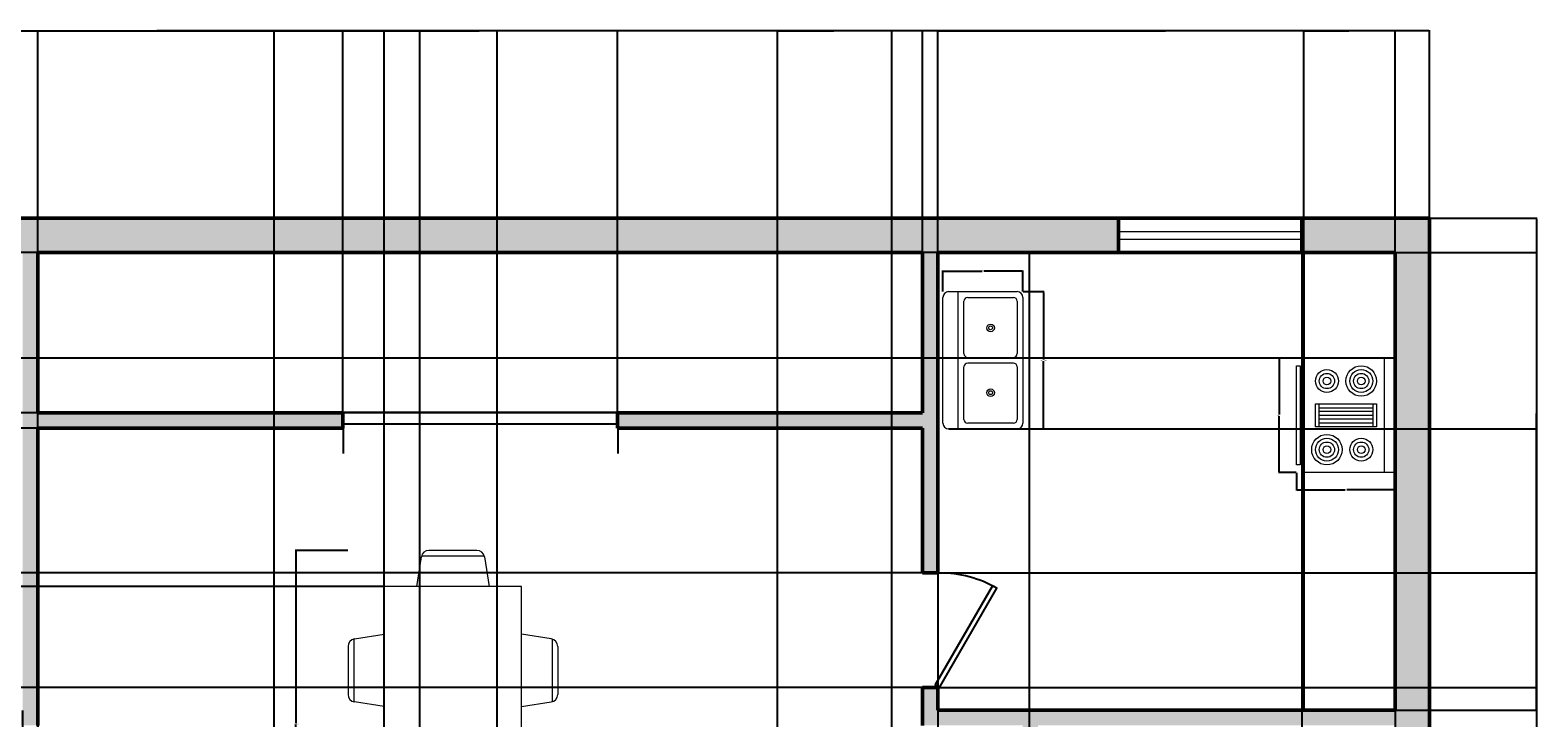
# Model space of a CAD drawing. Units: inches. Extents: x 1869 to 2483, y 2084 to 2479.
# Tile 7 of 7: x 2088 to 2483, y 2299 to 2479. Entities that reach past the tile are written whole.
import ezdxf

# ---------------------------------------------------------------- set-up
doc = ezdxf.new("R2010")
doc.units = ezdxf.units.IN
for name, color, linetype, lineweight in [('A-ANNO-DIMS', 2, 'Continuous', 18), ('A-DOOR', 3, 'Continuous', 25), ('A-EQPM', 8, 'Continuous', 18), ('A-FLOR-CASE', 9, 'Continuous', 25), ('A-FLOR-FIXT', 9, 'Continuous', 18), ('A-FURN', 8, 'Continuous', 18), ('A-GLAZ', 4, 'Continuous', 18), ('A-WALL', 7, 'Continuous', 50)]:
    doc.layers.add(name, color=color, linetype=linetype, lineweight=lineweight)
doc.layers.add('A-WALL-PATT', color=18, linetype='Continuous', lineweight=13, true_color=0x000000)
doc.styles.get("Standard").update_dxf_attribs({"font": 'arial.ttf'})
doc.dimstyles.get("Standard").update_dxf_attribs({"dimtxt": 0.18, "dimasz": 0.18, "dimexe": 0.18, "dimexo": 0.0625, "dimgap": 0.09, "dimtad": 0, "dimtih": 1, "dimtoh": 1, "dimdec": 4, "dimzin": 0, "dimdsep": 46, "dimtxsty": 'Standard', "dimcen": 0.09, "dimadec": 0, "dimazin": 0, "dimtfac": 1, "dimtdec": 4, "dimtofl": 0, "dimtmove": 0, "dimatfit": 3, "dimfxl": 1, "dimtolj": 1, "dimtzin": 0, "dimarcsym": 0})

# ---------------------------------------------------------------- blocks, each defined once
blk = doc.blocks.new('Dining Set - 36 x 72 in.')
for p, q in [((-22.26, 25.81), (-23.48, 18)), ((-22.23, 26), (-5.76, 26)), ((-20.29, 27.5), (-7.71, 27.5)), ((-4.52, 18), (-5.74, 25.81)), ((5.74, 25.81), (4.52, 18)), ((5.77, 26), (22.24, 26)), ((7.71, 27.5), (20.29, 27.5)), ((23.48, 18), (22.26, 25.81)), ((36, 18), (-36, 18)), ((-36, 18), (-36, -18)), ((36, -18), (36, 18)), ((-44, 8.23), (-44, -8.24)), ((-43.81, 8.26), (-36, 9.48)), ((43.81, 8.26), (36, 9.48)), ((44, 8.23), (44, -8.24)), ((-45.5, 6.29), (-45.5, -6.29)), ((45.5, 6.29), (45.5, -6.29)), ((-36, -9.48), (-43.81, -8.26)), ((36, -9.48), (43.81, -8.26)), ((-36, -18), (36, -18)), ((-22.26, -25.81), (-23.48, -18)), ((-4.52, -18), (-5.74, -25.81)), ((5.74, -25.81), (4.52, -18)), ((23.48, -18), (22.26, -25.81)), ((-22.23, -26), (-5.76, -26)), ((-20.29, -27.5), (-7.71, -27.5)), ((5.77, -26), (22.24, -26)), ((7.71, -27.5), (20.29, -27.5))]:
    blk.add_line(p, q)
for centre, start, end in [((-20.29, 25.5), 90, 171.1198), ((-7.71, 25.5), 8.881, 90), ((7.71, 25.5), 90, 171.1198), ((20.29, 25.5), 8.881, 90), ((-43.5, 6.29), 98.8806, 180), ((43.5, 6.29), 0, 81.1194), ((-43.5, -6.29), 180, 261.1194), ((43.5, -6.29), 278.8806, 0), ((-20.29, -25.5), 188.8802, 270), ((-7.71, -25.5), 270, 351.1191), ((7.71, -25.5), 188.8802, 270), ((20.29, -25.5), 270, 351.1191)]:
    blk.add_arc(centre, 2, start, end)
blk = doc.blocks.new('Range-Oven - 30 in top')
for p, q in [((0, -3), (30, -3)), ((12, -6), (18, -6)), ((13, -20), (13, -6)), ((14, -6), (14, -20)), ((15, -20), (15, -6)), ((16, -6), (16, -20)), ((17, -20), (17, -6)), ((18, -20), (12, -20)), ((6, -24), (6, -25)), ((8, -25), (8, -24)), ((22, -25), (22, -24)), ((24, -24), (24, -25))]:
    blk.add_line(p, q)
for points in [[(0, -24), (0, 0), (30, 0), (30, -24)], [(12, -21), (12, -5), (18, -5), (18, -21)], [(2, -26), (2, -25), (28, -25), (28, -26)]]:
    blk.add_lwpolyline(points, close=True)
for centre, radius in [((6, -9), 4), ((6, -9), 3), ((6, -9), 2), ((24, -9), 3), ((24, -9), 2), ((6, -9), 1), ((24, -9), 1), ((6, -18), 3), ((24, -18), 4), ((24, -18), 3), ((6, -18), 2), ((6, -18), 1), ((24, -18), 2), ((24, -18), 1)]:
    blk.add_circle(centre, radius)
blk = doc.blocks.new('Sink-double - 36 in top')
for p, q in [((-18, -4), (18, -4)), ((-0.75, -18.5), (-0.75, -6.5)), ((0.75, -6.5), (0.75, -18.5))]:
    blk.add_line(p, q)
for points in [[(-16.5, 0), (16.5, 0)], [(-18, -19.5), (-18, -1.5)], [(18, -1.5), (18, -19.5)], [(-16.5, -18.5), (-16.5, -6.5)], [(-15.5, -5.5), (-1.75, -5.5)], [(1.75, -5.5), (15.5, -5.5)], [(16.5, -6.5), (16.5, -18.5)], [(-1.75, -19.5), (-15.5, -19.5)], [(15.5, -19.5), (1.75, -19.5)], [(16.5, -21), (-16.5, -21)]]:
    blk.add_lwpolyline(points)
for centre, radius in [((-8.5, -12.5), 1), ((8.5, -12.5), 1), ((-8.5, -12.5), 0.5), ((8.5, -12.5), 0.5)]:
    blk.add_circle(centre, radius)
for centre, radius, start, end in [((-16.5, -1.5), 1.5, 90, 180), ((16.5, -1.5), 1.5, 0, 90), ((-15.5, -6.5), 1, 90, 180), ((-1.75, -6.5), 1, 0, 90), ((1.75, -6.5), 1, 90, 180), ((15.5, -6.5), 1, 0, 90), ((-16.5, -19.5), 1.5, 180, 270), ((-15.5, -18.5), 1, 180, 270), ((-1.75, -18.5), 1, 270, 0), ((1.75, -18.5), 1, 180, 270), ((15.5, -18.5), 1, 270, 0), ((16.5, -19.5), 1.5, 270, 0)]:
    blk.add_arc(centre, radius, start, end)
blk = doc.blocks.new('*U11')
for p, q in [((0, 0), (0, -6)), ((40, 0), (40, -6))]:
    blk.add_line(p, q)
blk.add_lwpolyline([(0, 0), (40, 0), (40, -1.75), (0, -1.75)], close=True)
blk = doc.blocks.new('*U12')
for p, q in [((0, 0), (0, -6)), ((-40, 0), (-40, -6))]:
    blk.add_line(p, q)
blk.add_lwpolyline([(0, 0), (-34.64, 20), (-35.52, 18.48), (-0.88, -1.52)], close=True)
blk.add_arc((0, 0), 40, 150, 180)
blk = doc.blocks.new('WIN-GLAZING-48IN')
for p, q in [((0, 2), (48, 2)), ((0, 0), (48, 0))]:
    blk.add_line(p, q)
blk = doc.blocks.new('*D29')
at = {"layer": 'A-ANNO-DIMS', "color": 0, "lineweight": -2, "transparency": 16777216}
for p, q in [((2171.37, 2342.65), (2157.61, 2342.65)), ((2157.79, 2342.47), (2157.79, 2297.33)), ((2157.79, 2251.83), (2157.79, 2296.97)), ((2171.37, 2251.65), (2157.61, 2251.65))]:
    blk.add_line(p, q, dxfattribs=at)
at = {"layer": 'A-ANNO-DIMS', "color": 0, "transparency": 16777216}
for points in [[(2157.76, 2342.47), (2157.82, 2342.47), (2157.79, 2342.65)], [(2157.76, 2251.83), (2157.82, 2251.83), (2157.79, 2251.65)]]:
    blk.add_solid(points, dxfattribs=at)
at = {"layer": 'Defpoints', "color": 0, "transparency": 16777216}
for p in [(2171.44, 2342.65), (2157.79, 2251.65), (2171.44, 2251.65)]:
    blk.add_point(p, dxfattribs=at)
at = {"layer": 'A-ANNO-DIMS', "color": 0, "transparency": 16777216, "insert": (2157.79, 2297.15), "char_height": 0.18, "attachment_point": 5}
blk.add_mtext('\\A1;DINING SET 91', dxfattribs=at)
blk = doc.blocks.new('*D31')
at = {"layer": 'A-ANNO-DIMS', "color": 0, "lineweight": -2, "transparency": 16777216}
for p, q in [((2420.08, 2393.06), (2415.46, 2393.06)), ((2415.64, 2392.88), (2415.64, 2378.24)), ((2415.64, 2363.24), (2415.64, 2377.87)), ((2420.08, 2363.06), (2415.46, 2363.06))]:
    blk.add_line(p, q, dxfattribs=at)
at = {"layer": 'A-ANNO-DIMS', "color": 0, "transparency": 16777216}
for points in [[(2415.61, 2392.88), (2415.67, 2392.88), (2415.64, 2393.06)], [(2415.61, 2363.24), (2415.67, 2363.24), (2415.64, 2363.06)]]:
    blk.add_solid(points, dxfattribs=at)
at = {"layer": 'Defpoints', "color": 0, "transparency": 16777216}
for p in [(2420.14, 2393.06), (2415.64, 2363.06), (2420.14, 2363.06)]:
    blk.add_point(p, dxfattribs=at)
at = {"layer": 'A-ANNO-DIMS', "color": 0, "transparency": 16777216, "insert": (2415.64, 2378.06), "char_height": 0.18, "attachment_point": 5}
blk.add_mtext('\\A1;RANGE 30', dxfattribs=at)
blk = doc.blocks.new('*D32')
at = {"layer": 'A-ANNO-DIMS', "color": 0, "lineweight": -2, "transparency": 16777216}
for p, q in [((2420.14, 2362.99), (2420.14, 2358.38)), ((2446.14, 2362.99), (2446.14, 2358.38)), ((2420.32, 2358.56), (2432.92, 2358.56)), ((2445.96, 2358.56), (2433.36, 2358.56))]:
    blk.add_line(p, q, dxfattribs=at)
at = {"layer": 'A-ANNO-DIMS', "color": 0, "transparency": 16777216}
for points in [[(2420.32, 2358.59), (2420.32, 2358.53), (2420.14, 2358.56)], [(2445.96, 2358.59), (2445.96, 2358.53), (2446.14, 2358.56)]]:
    blk.add_solid(points, dxfattribs=at)
at = {"layer": 'Defpoints', "color": 0, "transparency": 16777216}
for p in [(2420.14, 2363.06), (2446.14, 2363.06), (2446.14, 2358.56)]:
    blk.add_point(p, dxfattribs=at)
at = {"layer": 'A-ANNO-DIMS', "color": 0, "transparency": 16777216, "insert": (2433.14, 2358.56), "char_height": 0.18, "attachment_point": 5}
blk.add_mtext('\\A1;26', dxfattribs=at)
blk = doc.blocks.new('*D33')
at = {"layer": 'A-ANNO-DIMS', "color": 0, "lineweight": -2, "transparency": 16777216}
for p, q in [((2348.5, 2410.49), (2354.02, 2410.49)), ((2353.84, 2410.31), (2353.84, 2392.67)), ((2353.84, 2374.67), (2353.84, 2392.3)), ((2348.5, 2374.49), (2354.02, 2374.49))]:
    blk.add_line(p, q, dxfattribs=at)
at = {"layer": 'A-ANNO-DIMS', "color": 0, "transparency": 16777216}
for points in [[(2353.81, 2410.31), (2353.87, 2410.31), (2353.84, 2410.49)], [(2353.81, 2374.67), (2353.87, 2374.67), (2353.84, 2374.49)]]:
    blk.add_solid(points, dxfattribs=at)
at = {"layer": 'Defpoints', "color": 0, "transparency": 16777216}
for p in [(2348.44, 2410.49), (2353.84, 2410.49), (2348.44, 2374.49)]:
    blk.add_point(p, dxfattribs=at)
at = {"layer": 'A-ANNO-DIMS', "color": 0, "transparency": 16777216, "insert": (2353.84, 2392.49), "char_height": 0.18, "attachment_point": 5}
blk.add_mtext('\\A1;DOUBLE SINK 36', dxfattribs=at)
blk = doc.blocks.new('*D34')
at = {"layer": 'A-ANNO-DIMS', "color": 0, "lineweight": -2, "transparency": 16777216}
for p, q in [((2327.44, 2410.55), (2327.44, 2416.07)), ((2327.62, 2415.89), (2337.74, 2415.89)), ((2348.26, 2415.89), (2338.14, 2415.89)), ((2348.44, 2410.55), (2348.44, 2416.07))]:
    blk.add_line(p, q, dxfattribs=at)
at = {"layer": 'A-ANNO-DIMS', "color": 0, "transparency": 16777216}
for points in [[(2327.62, 2415.92), (2327.62, 2415.86), (2327.44, 2415.89)], [(2348.26, 2415.92), (2348.26, 2415.86), (2348.44, 2415.89)]]:
    blk.add_solid(points, dxfattribs=at)
at = {"layer": 'Defpoints', "color": 0, "transparency": 16777216}
for p in [(2327.44, 2415.89), (2327.44, 2410.49), (2348.44, 2410.49)]:
    blk.add_point(p, dxfattribs=at)
at = {"layer": 'A-ANNO-DIMS', "color": 0, "transparency": 16777216, "insert": (2337.94, 2415.89), "char_height": 0.18, "attachment_point": 5}
blk.add_mtext('\\A1;21', dxfattribs=at)
blk = doc.blocks.new('*D37')
at = {"layer": 'A-ANNO-DIMS', "color": 0, "lineweight": -2, "transparency": 16777216}
for p, q in [((2090.08, 2420.79), (2090.08, 2479.07)), ((2322.08, 2420.79), (2322.08, 2479.07)), ((2090.26, 2478.89), (2205.79, 2478.89)), ((2321.9, 2478.89), (2206.37, 2478.89))]:
    blk.add_line(p, q, dxfattribs=at)
at = {"layer": 'A-ANNO-DIMS', "color": 0, "transparency": 16777216}
for points in [[(2090.26, 2478.92), (2090.26, 2478.86), (2090.08, 2478.89)], [(2321.9, 2478.92), (2321.9, 2478.86), (2322.08, 2478.89)]]:
    blk.add_solid(points, dxfattribs=at)
at = {"layer": 'Defpoints', "color": 0, "transparency": 16777216}
for p in [(2322.08, 2478.89), (2090.08, 2420.72), (2322.08, 2420.72)]:
    blk.add_point(p, dxfattribs=at)
at = {"layer": 'A-ANNO-DIMS', "color": 0, "transparency": 16777216, "insert": (2206.08, 2478.89), "char_height": 0.18, "attachment_point": 5}
blk.add_mtext('\\A1;232', dxfattribs=at)
blk = doc.blocks.new('*D38')
at = {"layer": 'A-ANNO-DIMS', "color": 0, "lineweight": -2, "transparency": 16777216}
for p, q in [((2326.08, 2420.79), (2326.08, 2479.07)), ((2446.08, 2420.79), (2446.08, 2479.07)), ((2326.26, 2478.89), (2385.8, 2478.89)), ((2445.9, 2478.89), (2386.36, 2478.89))]:
    blk.add_line(p, q, dxfattribs=at)
at = {"layer": 'A-ANNO-DIMS', "color": 0, "transparency": 16777216}
for points in [[(2326.26, 2478.92), (2326.26, 2478.86), (2326.08, 2478.89)], [(2445.9, 2478.92), (2445.9, 2478.86), (2446.08, 2478.89)]]:
    blk.add_solid(points, dxfattribs=at)
at = {"layer": 'Defpoints', "color": 0, "transparency": 16777216}
for p in [(2446.08, 2478.89), (2326.08, 2420.72), (2446.08, 2420.72)]:
    blk.add_point(p, dxfattribs=at)
at = {"layer": 'A-ANNO-DIMS', "color": 0, "transparency": 16777216, "insert": (2386.08, 2478.89), "char_height": 0.18, "attachment_point": 5}
blk.add_mtext('\\A1;120', dxfattribs=at)
blk = doc.blocks.new('*D39')
at = {"layer": 'A-ANNO-DIMS', "color": 0, "lineweight": -2, "transparency": 16777216}
for p, q in [((2446.14, 2420.72), (2483.26, 2420.72)), ((2483.08, 2420.54), (2483.08, 2360.91)), ((2483.08, 2300.9), (2483.08, 2360.54)), ((2446.14, 2300.72), (2483.26, 2300.72))]:
    blk.add_line(p, q, dxfattribs=at)
at = {"layer": 'A-ANNO-DIMS', "color": 0, "transparency": 16777216}
for points in [[(2483.05, 2420.54), (2483.11, 2420.54), (2483.08, 2420.72)], [(2483.05, 2300.9), (2483.11, 2300.9), (2483.08, 2300.72)]]:
    blk.add_solid(points, dxfattribs=at)
at = {"layer": 'Defpoints', "color": 0, "transparency": 16777216}
for p in [(2446.08, 2420.72), (2483.08, 2420.72), (2446.08, 2300.72)]:
    blk.add_point(p, dxfattribs=at)
at = {"layer": 'A-ANNO-DIMS', "color": 0, "transparency": 16777216, "insert": (2483.08, 2360.72), "char_height": 0.18, "attachment_point": 5}
blk.add_mtext('\\A1;120', dxfattribs=at)
blk = doc.blocks.new('*D47')
at = {"layer": 'A-ANNO-DIMS', "color": 0, "lineweight": -2, "transparency": 16777216}
for p, q in [((2322.02, 2420.72), (1868.9, 2420.72)), ((1869.08, 2420.54), (1869.08, 2399.9)), ((1869.08, 2378.9), (1869.08, 2399.54)), ((2322.02, 2378.72), (1868.9, 2378.72))]:
    blk.add_line(p, q, dxfattribs=at)
at = {"layer": 'A-ANNO-DIMS', "color": 0, "transparency": 16777216}
for points in [[(1869.05, 2420.54), (1869.11, 2420.54), (1869.08, 2420.72)], [(1869.05, 2378.9), (1869.11, 2378.9), (1869.08, 2378.72)]]:
    blk.add_solid(points, dxfattribs=at)
at = {"layer": 'Defpoints', "color": 0, "transparency": 16777216}
for p in [(1869.08, 2420.72), (2322.08, 2420.72), (2322.08, 2378.72)]:
    blk.add_point(p, dxfattribs=at)
at = {"layer": 'A-ANNO-DIMS', "color": 0, "transparency": 16777216, "insert": (1869.08, 2399.72), "char_height": 0.18, "attachment_point": 5}
blk.add_mtext('\\A1;42', dxfattribs=at)
blk = doc.blocks.new('*D52')
at = {"layer": 'A-ANNO-DIMS', "color": 0, "lineweight": -2, "transparency": 16777216}
for p, q in [((2421.52, 2420.66), (2421.52, 2083.54)), ((2446.08, 2420.66), (2446.08, 2083.54)), ((2421.7, 2083.72), (2433.34, 2083.72)), ((2445.9, 2083.72), (2434.27, 2083.72))]:
    blk.add_line(p, q, dxfattribs=at)
at = {"layer": 'A-ANNO-DIMS', "color": 0, "transparency": 16777216}
for points in [[(2421.7, 2083.75), (2421.7, 2083.69), (2421.52, 2083.72)], [(2445.9, 2083.75), (2445.9, 2083.69), (2446.08, 2083.72)]]:
    blk.add_solid(points, dxfattribs=at)
at = {"layer": 'Defpoints', "color": 0, "transparency": 16777216}
for p in [(2421.52, 2420.72), (2446.08, 2420.72), (2446.08, 2083.72)]:
    blk.add_point(p, dxfattribs=at)
at = {"layer": 'A-ANNO-DIMS', "color": 0, "transparency": 16777216, "insert": (2433.8, 2083.72), "char_height": 0.18, "attachment_point": 5}
blk.add_mtext('\\A1;24.555', dxfattribs=at)
blk = doc.blocks.new('*D55')
at = {"layer": 'A-ANNO-DIMS', "color": 0, "lineweight": -2, "transparency": 16777216}
for p, q in [((2090.08, 2120.79), (2090.08, 2479.07)), ((2152.08, 2120.79), (2152.08, 2479.07)), ((2090.26, 2478.89), (2120.86, 2478.89)), ((2151.9, 2478.89), (2121.3, 2478.89))]:
    blk.add_line(p, q, dxfattribs=at)
at = {"layer": 'A-ANNO-DIMS', "color": 0, "transparency": 16777216}
for points in [[(2090.26, 2478.92), (2090.26, 2478.86), (2090.08, 2478.89)], [(2151.9, 2478.92), (2151.9, 2478.86), (2152.08, 2478.89)]]:
    blk.add_solid(points, dxfattribs=at)
at = {"layer": 'Defpoints', "color": 0, "transparency": 16777216}
for p in [(2152.08, 2478.89), (2090.08, 2120.72), (2152.08, 2120.72)]:
    blk.add_point(p, dxfattribs=at)
at = {"layer": 'A-ANNO-DIMS', "color": 0, "transparency": 16777216, "insert": (2121.08, 2478.89), "char_height": 0.18, "attachment_point": 5}
blk.add_mtext('\\A1;62', dxfattribs=at)
blk = doc.blocks.new('*D62')
at = {"layer": 'A-ANNO-DIMS', "color": 0, "lineweight": -2, "transparency": 16777216}
for p, q in [((2322.02, 2336.72), (1868.9, 2336.72)), ((1869.08, 2336.54), (1869.08, 2321.91)), ((1869.08, 2306.9), (1869.08, 2321.54)), ((2322.02, 2306.72), (1868.9, 2306.72))]:
    blk.add_line(p, q, dxfattribs=at)
at = {"layer": 'A-ANNO-DIMS', "color": 0, "transparency": 16777216}
for points in [[(1869.05, 2336.54), (1869.11, 2336.54), (1869.08, 2336.72)], [(1869.05, 2306.9), (1869.11, 2306.9), (1869.08, 2306.72)]]:
    blk.add_solid(points, dxfattribs=at)
at = {"layer": 'Defpoints', "color": 0, "transparency": 16777216}
for p in [(1869.08, 2336.72), (2322.08, 2336.72), (2322.08, 2306.72)]:
    blk.add_point(p, dxfattribs=at)
at = {"layer": 'A-ANNO-DIMS', "color": 0, "transparency": 16777216, "insert": (1869.08, 2321.72), "char_height": 0.18, "attachment_point": 5}
blk.add_mtext('\\A1;30', dxfattribs=at)
blk = doc.blocks.new('*D64')
at = {"layer": 'A-ANNO-DIMS', "color": 0, "lineweight": -2, "transparency": 16777216}
for p, q in [((2284.08, 2236.79), (2284.08, 2479.07)), ((2314.08, 2236.79), (2314.08, 2479.07)), ((2284.26, 2478.89), (2298.86, 2478.89)), ((2313.9, 2478.89), (2299.3, 2478.89))]:
    blk.add_line(p, q, dxfattribs=at)
at = {"layer": 'A-ANNO-DIMS', "color": 0, "transparency": 16777216}
for points in [[(2284.26, 2478.92), (2284.26, 2478.86), (2284.08, 2478.89)], [(2313.9, 2478.92), (2313.9, 2478.86), (2314.08, 2478.89)]]:
    blk.add_solid(points, dxfattribs=at)
at = {"layer": 'Defpoints', "color": 0, "transparency": 16777216}
for p in [(2314.08, 2478.89), (2284.08, 2236.72), (2314.08, 2236.72)]:
    blk.add_point(p, dxfattribs=at)
at = {"layer": 'A-ANNO-DIMS', "color": 0, "transparency": 16777216, "insert": (2299.08, 2478.89), "char_height": 0.18, "attachment_point": 5}
blk.add_mtext('\\A1;30', dxfattribs=at)
blk = doc.blocks.new('*D70')
at = {"layer": 'A-ANNO-DIMS', "color": 0, "lineweight": -2, "transparency": 16777216}
for p, q in [((2170.08, 2378.79), (2170.08, 2479.07)), ((2242.08, 2378.79), (2242.08, 2479.07)), ((2170.26, 2478.89), (2205.86, 2478.89)), ((2241.9, 2478.89), (2206.3, 2478.89))]:
    blk.add_line(p, q, dxfattribs=at)
at = {"layer": 'A-ANNO-DIMS', "color": 0, "transparency": 16777216}
for points in [[(2170.26, 2478.92), (2170.26, 2478.86), (2170.08, 2478.89)], [(2241.9, 2478.92), (2241.9, 2478.86), (2242.08, 2478.89)]]:
    blk.add_solid(points, dxfattribs=at)
at = {"layer": 'Defpoints', "color": 0, "transparency": 16777216}
for p in [(2242.08, 2478.89), (2170.08, 2378.72), (2242.08, 2378.72)]:
    blk.add_point(p, dxfattribs=at)
at = {"layer": 'A-ANNO-DIMS', "color": 0, "transparency": 16777216, "insert": (2206.08, 2478.89), "char_height": 0.18, "attachment_point": 5}
blk.add_mtext('\\A1;72', dxfattribs=at)
blk = doc.blocks.new('*D71')
at = {"layer": 'A-ANNO-DIMS', "color": 0, "lineweight": -2, "transparency": 16777216}
for p, q in [((2090.08, 2378.79), (2090.08, 2479.07)), ((2170.08, 2378.79), (2170.08, 2479.07)), ((2090.26, 2478.89), (2129.86, 2478.89)), ((2169.9, 2478.89), (2130.3, 2478.89))]:
    blk.add_line(p, q, dxfattribs=at)
at = {"layer": 'A-ANNO-DIMS', "color": 0, "transparency": 16777216}
for points in [[(2090.26, 2478.92), (2090.26, 2478.86), (2090.08, 2478.89)], [(2169.9, 2478.92), (2169.9, 2478.86), (2170.08, 2478.89)]]:
    blk.add_solid(points, dxfattribs=at)
at = {"layer": 'Defpoints', "color": 0, "transparency": 16777216}
for p in [(2170.08, 2478.89), (2090.08, 2378.72), (2170.08, 2378.72)]:
    blk.add_point(p, dxfattribs=at)
at = {"layer": 'A-ANNO-DIMS', "color": 0, "transparency": 16777216, "insert": (2130.08, 2478.89), "char_height": 0.18, "attachment_point": 5}
blk.add_mtext('\\A1;80', dxfattribs=at)
blk = doc.blocks.new('*D72')
at = {"layer": 'A-ANNO-DIMS', "color": 0, "lineweight": -2, "transparency": 16777216}
for p, q in [((2086.08, 2300.66), (2086.08, 2083.54)), ((2090.08, 2296.66), (2090.08, 2083.54)), ((2086.26, 2083.72), (2087.93, 2083.72)), ((2089.9, 2083.72), (2088.23, 2083.72))]:
    blk.add_line(p, q, dxfattribs=at)
at = {"layer": 'A-ANNO-DIMS', "color": 0, "transparency": 16777216}
for points in [[(2086.26, 2083.75), (2086.26, 2083.69), (2086.08, 2083.72)], [(2089.9, 2083.75), (2089.9, 2083.69), (2090.08, 2083.72)]]:
    blk.add_solid(points, dxfattribs=at)
at = {"layer": 'Defpoints', "color": 0, "transparency": 16777216}
for p in [(2086.08, 2300.72), (2090.08, 2296.72), (2090.08, 2083.72)]:
    blk.add_point(p, dxfattribs=at)
at = {"layer": 'A-ANNO-DIMS', "color": 0, "transparency": 16777216, "insert": (2088.08, 2083.72), "char_height": 0.18, "attachment_point": 5}
blk.add_mtext('\\A1;4', dxfattribs=at)
blk = doc.blocks.new('*D75')
at = {"layer": 'A-ANNO-DIMS', "color": 0, "lineweight": -2, "transparency": 16777216}
for p, q in [((1897.08, 2429.79), (1897.08, 2479.07)), ((2455.08, 2429.79), (2455.08, 2479.07)), ((1897.26, 2478.89), (2175.79, 2478.89)), ((2454.9, 2478.89), (2176.37, 2478.89))]:
    blk.add_line(p, q, dxfattribs=at)
at = {"layer": 'A-ANNO-DIMS', "color": 0, "transparency": 16777216}
for points in [[(1897.26, 2478.92), (1897.26, 2478.86), (1897.08, 2478.89)], [(2454.9, 2478.92), (2454.9, 2478.86), (2455.08, 2478.89)]]:
    blk.add_solid(points, dxfattribs=at)
at = {"layer": 'Defpoints', "color": 0, "transparency": 16777216}
for p in [(2455.08, 2478.89), (1897.08, 2429.72), (2455.08, 2429.72)]:
    blk.add_point(p, dxfattribs=at)
at = {"layer": 'A-ANNO-DIMS', "color": 0, "transparency": 16777216, "insert": (2176.08, 2478.89), "char_height": 0.18, "attachment_point": 5}
blk.add_mtext('\\A1;558', dxfattribs=at)
blk = doc.blocks.new('*D76')
at = {"layer": 'A-ANNO-DIMS', "color": 0, "lineweight": -2, "transparency": 16777216}
for p, q in [((2455.14, 2429.72), (2483.26, 2429.72)), ((2483.08, 2429.54), (2483.08, 2270.91)), ((2483.08, 2111.9), (2483.08, 2270.54)), ((2455.14, 2111.72), (2483.26, 2111.72))]:
    blk.add_line(p, q, dxfattribs=at)
at = {"layer": 'A-ANNO-DIMS', "color": 0, "transparency": 16777216}
for points in [[(2483.05, 2429.54), (2483.11, 2429.54), (2483.08, 2429.72)], [(2483.05, 2111.9), (2483.11, 2111.9), (2483.08, 2111.72)]]:
    blk.add_solid(points, dxfattribs=at)
at = {"layer": 'Defpoints', "color": 0, "transparency": 16777216}
for p in [(2455.08, 2429.72), (2483.08, 2429.72), (2455.08, 2111.72)]:
    blk.add_point(p, dxfattribs=at)
at = {"layer": 'A-ANNO-DIMS', "color": 0, "transparency": 16777216, "insert": (2483.08, 2270.72), "char_height": 0.18, "attachment_point": 5}
blk.add_mtext('\\A1;318', dxfattribs=at)
blk = doc.blocks.new('*D77')
at = {"layer": 'A-ANNO-DIMS', "color": 0, "lineweight": -2, "transparency": 16777216}
for p, q in [((2326.08, 2336.66), (2326.08, 2083.54)), ((2350.08, 2336.66), (2350.08, 2083.54)), ((2326.26, 2083.72), (2337.86, 2083.72)), ((2349.9, 2083.72), (2338.3, 2083.72))]:
    blk.add_line(p, q, dxfattribs=at)
at = {"layer": 'A-ANNO-DIMS', "color": 0, "transparency": 16777216}
for points in [[(2326.26, 2083.75), (2326.26, 2083.69), (2326.08, 2083.72)], [(2349.9, 2083.75), (2349.9, 2083.69), (2350.08, 2083.72)]]:
    blk.add_solid(points, dxfattribs=at)
at = {"layer": 'Defpoints', "color": 0, "transparency": 16777216}
for p in [(2326.08, 2336.72), (2350.08, 2336.72), (2350.08, 2083.72)]:
    blk.add_point(p, dxfattribs=at)
at = {"layer": 'A-ANNO-DIMS', "color": 0, "transparency": 16777216, "insert": (2338.08, 2083.72), "char_height": 0.18, "attachment_point": 5}
blk.add_mtext('\\A1;24', dxfattribs=at)
blk = doc.blocks.new('*D78')
at = {"layer": 'A-ANNO-DIMS', "color": 0, "lineweight": -2, "transparency": 16777216}
for p, q in [((2350.14, 2420.72), (2483.26, 2420.72)), ((2483.08, 2420.54), (2483.08, 2378.91)), ((2483.08, 2336.9), (2483.08, 2378.54)), ((2350.14, 2336.72), (2483.26, 2336.72))]:
    blk.add_line(p, q, dxfattribs=at)
at = {"layer": 'A-ANNO-DIMS', "color": 0, "transparency": 16777216}
for points in [[(2483.05, 2420.54), (2483.11, 2420.54), (2483.08, 2420.72)], [(2483.05, 2336.9), (2483.11, 2336.9), (2483.08, 2336.72)]]:
    blk.add_solid(points, dxfattribs=at)
at = {"layer": 'Defpoints', "color": 0, "transparency": 16777216}
for p in [(2350.08, 2420.72), (2483.08, 2420.72), (2350.08, 2336.72)]:
    blk.add_point(p, dxfattribs=at)
at = {"layer": 'A-ANNO-DIMS', "color": 0, "transparency": 16777216, "insert": (2483.08, 2378.72), "char_height": 0.18, "attachment_point": 5}
blk.add_mtext('\\A1;84', dxfattribs=at)
blk = doc.blocks.new('*D79')
at = {"layer": 'A-ANNO-DIMS', "color": 0, "lineweight": -2, "transparency": 16777216}
for p, q in [((2326.14, 2306.72), (2483.26, 2306.72)), ((2483.08, 2306.54), (2483.08, 2303.91)), ((2483.08, 2300.9), (2483.08, 2303.54)), ((2326.14, 2300.72), (2483.26, 2300.72))]:
    blk.add_line(p, q, dxfattribs=at)
at = {"layer": 'A-ANNO-DIMS', "color": 0, "transparency": 16777216}
for points in [[(2483.05, 2306.54), (2483.11, 2306.54), (2483.08, 2306.72)], [(2483.05, 2300.9), (2483.11, 2300.9), (2483.08, 2300.72)]]:
    blk.add_solid(points, dxfattribs=at)
at = {"layer": 'Defpoints', "color": 0, "transparency": 16777216}
for p in [(2326.08, 2306.72), (2483.08, 2306.72), (2326.08, 2300.72)]:
    blk.add_point(p, dxfattribs=at)
at = {"layer": 'A-ANNO-DIMS', "color": 0, "transparency": 16777216, "insert": (2483.08, 2303.72), "char_height": 0.18, "attachment_point": 5}
blk.add_mtext('\\A1;6', dxfattribs=at)
blk = doc.blocks.new('*D88')
at = {"layer": 'A-ANNO-DIMS', "color": 0, "lineweight": -2, "transparency": 16777216}
for p, q in [((2422.08, 2300.79), (2422.08, 2479.07)), ((2446.08, 2300.79), (2446.08, 2479.07)), ((2422.26, 2478.89), (2433.86, 2478.89)), ((2445.9, 2478.89), (2434.3, 2478.89))]:
    blk.add_line(p, q, dxfattribs=at)
at = {"layer": 'A-ANNO-DIMS', "color": 0, "transparency": 16777216}
for points in [[(2422.26, 2478.92), (2422.26, 2478.86), (2422.08, 2478.89)], [(2445.9, 2478.92), (2445.9, 2478.86), (2446.08, 2478.89)]]:
    blk.add_solid(points, dxfattribs=at)
at = {"layer": 'Defpoints', "color": 0, "transparency": 16777216}
for p in [(2446.08, 2478.89), (2422.08, 2300.72), (2446.08, 2300.72)]:
    blk.add_point(p, dxfattribs=at)
at = {"layer": 'A-ANNO-DIMS', "color": 0, "transparency": 16777216, "insert": (2434.08, 2478.89), "char_height": 0.18, "attachment_point": 5}
blk.add_mtext('\\A1;24', dxfattribs=at)
blk = doc.blocks.new('*D91')
at = {"layer": 'A-ANNO-DIMS', "color": 0, "lineweight": -2, "transparency": 16777216}
for p, q in [((2190.29, 2192.37), (2190.29, 2479.07)), ((2210.52, 2192.37), (2210.52, 2479.07)), ((2190.47, 2478.89), (2199.94, 2478.89)), ((2210.34, 2478.89), (2200.87, 2478.89))]:
    blk.add_line(p, q, dxfattribs=at)
at = {"layer": 'A-ANNO-DIMS', "color": 0, "transparency": 16777216}
for points in [[(2190.47, 2478.92), (2190.47, 2478.86), (2190.29, 2478.89)], [(2210.34, 2478.92), (2210.34, 2478.86), (2210.52, 2478.89)]]:
    blk.add_solid(points, dxfattribs=at)
at = {"layer": 'Defpoints', "color": 0, "transparency": 16777216}
for p in [(2210.52, 2478.89), (2190.29, 2192.3), (2210.52, 2192.3)]:
    blk.add_point(p, dxfattribs=at)
at = {"layer": 'A-ANNO-DIMS', "color": 0, "transparency": 16777216, "insert": (2200.4, 2478.89), "char_height": 0.18, "attachment_point": 5}
blk.add_mtext('\\A1;20.236', dxfattribs=at)
blk = doc.blocks.new('*D94')
at = {"layer": 'A-ANNO-DIMS', "color": 0, "lineweight": -2, "transparency": 16777216}
for p, q in [((2170.02, 2374.72), (1868.9, 2374.72)), ((1869.08, 2374.54), (1869.08, 2354.12)), ((1869.08, 2333.33), (1869.08, 2353.75)), ((2180.87, 2333.15), (1868.9, 2333.15))]:
    blk.add_line(p, q, dxfattribs=at)
at = {"layer": 'A-ANNO-DIMS', "color": 0, "transparency": 16777216}
for points in [[(1869.05, 2374.54), (1869.11, 2374.54), (1869.08, 2374.72)], [(1869.05, 2333.33), (1869.11, 2333.33), (1869.08, 2333.15)]]:
    blk.add_solid(points, dxfattribs=at)
at = {"layer": 'Defpoints', "color": 0, "transparency": 16777216}
for p in [(2170.08, 2374.72), (1869.08, 2333.15), (2180.94, 2333.15)]:
    blk.add_point(p, dxfattribs=at)
at = {"layer": 'A-ANNO-DIMS', "color": 0, "transparency": 16777216, "insert": (1869.08, 2353.94), "char_height": 0.18, "attachment_point": 5}
blk.add_mtext('\\A1;41.575', dxfattribs=at)
blk = doc.blocks.new('*D95')
at = {"layer": 'A-ANNO-DIMS', "color": 0, "lineweight": -2, "transparency": 16777216}
for p, q in [((2090.08, 2296.79), (2090.08, 2479.07)), ((2180.94, 2261.21), (2180.94, 2479.07)), ((2090.26, 2478.89), (2135.11, 2478.89)), ((2180.76, 2478.89), (2135.9, 2478.89))]:
    blk.add_line(p, q, dxfattribs=at)
at = {"layer": 'A-ANNO-DIMS', "color": 0, "transparency": 16777216}
for points in [[(2090.26, 2478.92), (2090.26, 2478.86), (2090.08, 2478.89)], [(2180.76, 2478.92), (2180.76, 2478.86), (2180.94, 2478.89)]]:
    blk.add_solid(points, dxfattribs=at)
at = {"layer": 'Defpoints', "color": 0, "transparency": 16777216}
for p in [(2180.94, 2478.89), (2090.08, 2296.72), (2180.94, 2261.15)]:
    blk.add_point(p, dxfattribs=at)
at = {"layer": 'A-ANNO-DIMS', "color": 0, "transparency": 16777216, "insert": (2135.51, 2478.89), "char_height": 0.18, "attachment_point": 5}
blk.add_mtext('\\A1;90.86', dxfattribs=at)
blk = doc.blocks.new('*D96')
at = {"layer": 'A-ANNO-DIMS', "color": 0, "lineweight": -2, "transparency": 16777216}
for p, q in [((2446.02, 2420.72), (1868.9, 2420.72)), ((1869.08, 2420.54), (1869.08, 2407.07)), ((1869.08, 2393.24), (1869.08, 2406.71)), ((2446.08, 2393.06), (1868.9, 2393.06))]:
    blk.add_line(p, q, dxfattribs=at)
at = {"layer": 'A-ANNO-DIMS', "color": 0, "transparency": 16777216}
for points in [[(1869.05, 2420.54), (1869.11, 2420.54), (1869.08, 2420.72)], [(1869.05, 2393.24), (1869.11, 2393.24), (1869.08, 2393.06)]]:
    blk.add_solid(points, dxfattribs=at)
at = {"layer": 'Defpoints', "color": 0, "transparency": 16777216}
for p in [(1869.08, 2420.72), (2446.08, 2420.72), (2446.14, 2393.06)]:
    blk.add_point(p, dxfattribs=at)
at = {"layer": 'A-ANNO-DIMS', "color": 0, "transparency": 16777216, "insert": (1869.08, 2406.89), "char_height": 0.18, "attachment_point": 5}
blk.add_mtext('\\A1;27.667', dxfattribs=at)
blk = doc.blocks.new('*D97')
at = {"layer": 'A-ANNO-DIMS', "color": 0, "lineweight": -2, "transparency": 16777216}
for p, q in [((2329, 2374.49), (2483.26, 2374.49)), ((2483.08, 2374.31), (2483.08, 2355.79)), ((2483.08, 2336.9), (2483.08, 2355.42)), ((2326.14, 2336.72), (2483.26, 2336.72))]:
    blk.add_line(p, q, dxfattribs=at)
at = {"layer": 'A-ANNO-DIMS', "color": 0, "transparency": 16777216}
for points in [[(2483.05, 2374.31), (2483.11, 2374.31), (2483.08, 2374.49)], [(2483.05, 2336.9), (2483.11, 2336.9), (2483.08, 2336.72)]]:
    blk.add_solid(points, dxfattribs=at)
at = {"layer": 'Defpoints', "color": 0, "transparency": 16777216}
for p in [(2328.94, 2374.49), (2483.08, 2374.49), (2326.08, 2336.72)]:
    blk.add_point(p, dxfattribs=at)
at = {"layer": 'A-ANNO-DIMS', "color": 0, "transparency": 16777216, "insert": (2483.08, 2355.61), "char_height": 0.18, "attachment_point": 5}
blk.add_mtext('\\A1;37.764', dxfattribs=at)

msp = doc.modelspace()

# ---------------------------------------------------------------- hatches: boundary and pattern name
at = {"layer": 'A-WALL-PATT'}
h = msp.add_hatch(color=256, dxfattribs=at)
h.dxf.hatch_style = 1
h.paths.add_polyline_path([(2373.5248, 2429.7235), (2046.5221, 2429.7235), (2046.5221, 2420.7235), (2086.0799, 2420.7235), (2086.0799, 2330.7235), (2086.0799, 2300.7235), (2080.0799, 2300.7235), (2080.0799, 2296.7235), (2090.0799, 2296.7235), (2090.0799, 2374.7235), (2170.0799, 2374.7235), (2170.0799, 2378.7235), (2090.0799, 2378.7235), (2090.0799, 2420.7235), (2322.0799, 2420.7235), (2322.0799, 2378.7235), (2242.0799, 2378.7235), (2242.0799, 2374.7235), (2322.0799, 2374.7235), (2322.0799, 2336.7235), (2326.0799, 2336.7235), (2326.0799, 2420.7235), (2373.5248, 2420.7235)])
h = msp.add_hatch(color=256, dxfattribs=at)
h.dxf.hatch_style = 1
h.paths.add_polyline_path([(2352.3982, 2296.7235), (2446.0799, 2296.7235), (2446.0799, 2252.0706), (2455.0799, 2252.0706), (2455.0799, 2429.7235), (2421.5248, 2429.7235), (2421.5248, 2420.7235), (2446.0799, 2420.7235), (2446.0799, 2300.7235), (2326.0799, 2300.7235), (2326.0799, 2306.7235), (2322.0799, 2306.7235), (2322.0799, 2296.7235), (2348.3982, 2296.7235), (2348.3982, 2272.7235), (2352.3982, 2272.7235)])

# ---------------------------------------------------------------- linework, layer by layer
at = {"layer": 'A-FLOR-CASE'}
for p, q in [((2350.0799, 2420.7235), (2350.0799, 2336.7235)), ((2422.0799, 2420.7235), (2422.0799, 2300.7235)), ((2326.0799, 2336.7235), (2350.0799, 2336.7235))]:
    msp.add_line(p, q, dxfattribs=at)
at = {"layer": 'A-WALL'}
for p, q in [((2373.5248, 2420.7235), (2373.5248, 2429.7235)), ((2421.5248, 2429.7235), (2421.5248, 2420.7235)), ((2090.0799, 2420.7235), (2322.0799, 2420.7235)), ((2090.0799, 2378.7235), (2090.0799, 2420.7235)), ((2322.0799, 2420.7235), (2322.0799, 2378.7235)), ((2322.0799, 2420.7235), (2322.0799, 2378.7235)), ((2326.0799, 2420.7235), (2326.0799, 2336.7235)), ((2326.0799, 2420.7235), (2446.0799, 2420.7235)), ((2446.0799, 2420.7235), (2446.0799, 2300.7235)), ((2090.0799, 2378.7235), (2170.0799, 2378.7235)), ((2170.0799, 2374.7235), (2170.0799, 2378.7235)), ((2242.0799, 2374.7235), (2242.0799, 2378.7235)), ((2242.0799, 2378.7235), (2322.0799, 2378.7235)), ((2090.0799, 2296.7235), (2090.0799, 2374.7235)), ((2090.0799, 2374.7235), (2170.0799, 2374.7235)), ((2242.0799, 2374.7235), (2322.0799, 2374.7235)), ((2322.0799, 2374.7235), (2322.0799, 2336.7235)), ((2326.0799, 2336.7235), (2322.0799, 2336.7235)), ((2326.0799, 2306.7235), (2322.0799, 2306.7235)), ((2322.0799, 2306.7235), (2322.0799, 2296.7235)), ((2326.0799, 2306.7235), (2326.0799, 2300.7235)), ((2326.0799, 2300.7235), (2446.0799, 2300.7235))]:
    msp.add_line(p, q, dxfattribs=at)
msp.add_lwpolyline([(2152.0799, 2111.7235), (1897.0799, 2111.7235), (1897.0799, 2429.7235), (2455.0799, 2429.7235), (2455.0799, 2111.7235), (2200.0799, 2111.7235)], dxfattribs=at)

# ---------------------------------------------------------------- block references
at = {"layer": 'A-DOOR', "xscale": 1.8, "yscale": 1.8, "zscale": 1.8}
msp.add_blockref('*U11', (2170.1966, 2378.8871), dxfattribs=at)
at = {"layer": 'A-DOOR', "xscale": 0.75, "yscale": 0.75, "zscale": 0.75, "rotation": 270}
msp.add_blockref('*U12', (2326.5799, 2306.7235), dxfattribs=at)
at = {"layer": 'A-EQPM', "rotation": 270}
msp.add_blockref('Range-Oven - 30 in top', (2446.143, 2393.0569), dxfattribs=at)
at = {"layer": 'A-FLOR-FIXT', "rotation": 90}
msp.add_blockref('Sink-double - 36 in top', (2327.4404, 2392.4879), dxfattribs=at)
at = {"layer": 'A-FURN', "rotation": 270}
msp.add_blockref('Dining Set - 36 x 72 in.', (2198.9372, 2297.1488), dxfattribs=at)
at = {"layer": 'A-GLAZ'}
msp.add_blockref('WIN-GLAZING-48IN', (2373.5247, 2424.224), dxfattribs=at)

# ---------------------------------------------------------------- dimensions: what is measured, and where the dimension line sits
at = {"layer": 'A-ANNO-DIMS'}
for base, p1, p2, override, picture, middle in [((2455.0799, 2478.8871), (1897.0799, 2429.7235), (2455.0799, 2429.7235), {"dimdec": 0, "dimlfac": 1, "dimrnd": 0, "dimzin": 0, "dimdsep": 46, "dimlunit": 2}, '*D75', (2176.0799, 2478.8871)), ((2322.0799, 2478.8871), (2090.0799, 2420.7235), (2322.0799, 2420.7235), {"dimdec": 0, "dimlfac": 1, "dimrnd": 0, "dimzin": 0, "dimdsep": 46, "dimlunit": 2}, '*D37', (2206.0799, 2478.8871)), ((2152.0799, 2478.8871), (2090.0799, 2120.7235), (2152.0799, 2120.7235), {"dimdec": 0, "dimlfac": 1, "dimrnd": 0, "dimzin": 0, "dimdsep": 46, "dimlunit": 2}, '*D55', (2121.0799, 2478.8871)), ((2170.0799, 2478.8871), (2090.0799, 2378.7235), (2170.0799, 2378.7235), {"dimdec": 0, "dimlfac": 1, "dimrnd": 0, "dimzin": 0, "dimdsep": 46, "dimlunit": 2}, '*D71', (2130.0799, 2478.8871)), ((2180.9372, 2478.8871), (2090.0799, 2296.7235), (2180.9372, 2261.1488), {"dimdec": 2, "dimlfac": 1, "dimrnd": 0, "dimzin": 0, "dimdsep": 46, "dimlunit": 2}, '*D95', (2135.5085, 2478.8871)), ((2242.0799, 2478.8871), (2170.0799, 2378.7235), (2242.0799, 2378.7235), {"dimdec": 0, "dimlfac": 1, "dimrnd": 0, "dimzin": 0, "dimdsep": 46, "dimlunit": 2}, '*D70', (2206.0799, 2478.8871)), ((2210.5231, 2478.8871), (2190.2869, 2192.3029), (2210.5231, 2192.3029), {"dimdec": 3, "dimlfac": 1, "dimrnd": 0, "dimzin": 0, "dimdsep": 46, "dimlunit": 2}, '*D91', (2200.405, 2478.8871)), ((2314.0799, 2478.8871), (2284.0799, 2236.7235), (2314.0799, 2236.7235), {"dimdec": 0, "dimlfac": 1, "dimrnd": 0, "dimzin": 0, "dimdsep": 46, "dimlunit": 2}, '*D64', (2299.0799, 2478.8871)), ((2446.0799, 2478.8871), (2326.0799, 2420.7235), (2446.0799, 2420.7235), {"dimdec": 0, "dimlfac": 1, "dimrnd": 0, "dimzin": 0, "dimdsep": 46, "dimlunit": 2}, '*D38', (2386.0799, 2478.8871)), ((2446.0799, 2478.8871), (2422.0799, 2300.7235), (2446.0799, 2300.7235), {"dimdec": 0, "dimlfac": 1, "dimrnd": 0, "dimzin": 0, "dimdsep": 46, "dimlunit": 2}, '*D88', (2434.0799, 2478.8871)), ((2446.0799, 2083.7235), (2421.5248, 2420.7235), (2446.0799, 2420.7235), {"dimdec": 3, "dimlfac": 1, "dimrnd": 0, "dimzin": 0, "dimdsep": 46, "dimlunit": 2}, '*D52', (2433.8023, 2083.7235)), ((2446.143, 2358.5569), (2420.143, 2363.0569), (2446.143, 2363.0569), {"dimdec": 0, "dimlfac": 1, "dimrnd": 0, "dimzin": 0, "dimdsep": 46, "dimlunit": 2}, '*D32', (2433.143, 2358.5569)), ((2350.0799, 2083.7235), (2326.0799, 2336.7235), (2350.0799, 2336.7235), {"dimdec": 0, "dimlfac": 1, "dimrnd": 0, "dimzin": 0, "dimdsep": 46, "dimlunit": 2}, '*D77', (2338.0799, 2083.7235)), ((2090.0799, 2083.7235), (2086.0799, 2300.7235), (2090.0799, 2296.7235), {"dimdec": 0, "dimlfac": 1, "dimrnd": 0, "dimzin": 0, "dimdsep": 46, "dimlunit": 2}, '*D72', (2088.0799, 2083.7235))]:
    dim = msp.add_linear_dim(base=base, p1=p1, p2=p2, dimstyle='Standard', override=override, dxfattribs=at)
    dim.commit()
    dim.dimension.update_dxf_attribs({"geometry": picture, "text_midpoint": middle})
for base, p1, p2, angle, override, picture, middle in [((2483.0799, 2429.7235), (2455.0799, 2111.7235), (2455.0799, 2429.7235), 90, {"dimdec": 0, "dimlfac": 1, "dimrnd": 0, "dimzin": 0, "dimdsep": 46, "dimlunit": 2}, '*D76', (2483.0799, 2270.7235)), ((1869.0799, 2420.7235), (2446.143, 2393.0569), (2446.0799, 2420.7235), 90, {"dimdec": 3, "dimlfac": 1, "dimrnd": 0, "dimzin": 0, "dimdsep": 46, "dimlunit": 2}, '*D96', (1869.0799, 2406.8902)), ((1869.0799, 2420.7235), (2322.0799, 2378.7235), (2322.0799, 2420.7235), 90, {"dimdec": 0, "dimlfac": 1, "dimrnd": 0, "dimzin": 0, "dimdsep": 46, "dimlunit": 2}, '*D47', (1869.0799, 2399.7235)), ((2483.0799, 2420.7235), (2350.0799, 2336.7235), (2350.0799, 2420.7235), 90, {"dimdec": 0, "dimlfac": 1, "dimrnd": 0, "dimzin": 0, "dimdsep": 46, "dimlunit": 2}, '*D78', (2483.0799, 2378.7235)), ((2483.0799, 2420.7235), (2446.0799, 2300.7235), (2446.0799, 2420.7235), 90, {"dimdec": 0, "dimlfac": 1, "dimrnd": 0, "dimzin": 0, "dimdsep": 46, "dimlunit": 2}, '*D39', (2483.0799, 2360.7235)), ((2327.4404, 2415.8879), (2348.4404, 2410.4879), (2327.4404, 2410.4879), 180, {"dimdec": 0, "dimlfac": 1, "dimrnd": 0, "dimzin": 0, "dimdsep": 46, "dimlunit": 2}, '*D34', (2337.9404, 2415.8879)), ((1869.0799, 2333.1488), (2170.0799, 2374.7235), (2180.9372, 2333.1488), 90, {"dimdec": 3, "dimlfac": 1, "dimrnd": 0, "dimzin": 0, "dimdsep": 46, "dimlunit": 2}, '*D94', (1869.0799, 2353.9361)), ((2483.0799, 2374.4879), (2326.0799, 2336.7235), (2328.9404, 2374.4879), 90, {"dimdec": 3, "dimlfac": 1, "dimrnd": 0, "dimzin": 0, "dimdsep": 46, "dimlunit": 2}, '*D97', (2483.0799, 2355.6057)), ((1869.0799, 2336.7235), (2322.0799, 2306.7235), (2322.0799, 2336.7235), 90, {"dimdec": 0, "dimlfac": 1, "dimrnd": 0, "dimzin": 0, "dimdsep": 46, "dimlunit": 2}, '*D62', (1869.0799, 2321.7235)), ((2483.0799, 2306.7235), (2326.0799, 2300.7235), (2326.0799, 2306.7235), 90, {"dimdec": 0, "dimlfac": 1, "dimrnd": 0, "dimzin": 0, "dimdsep": 46, "dimlunit": 2}, '*D79', (2483.0799, 2303.7235))]:
    dim = msp.add_linear_dim(base=base, p1=p1, p2=p2, angle=angle, dimstyle='Standard', override=override, dxfattribs=at)
    dim.commit()
    dim.dimension.update_dxf_attribs({"geometry": picture, "text_midpoint": middle})
for base, p1, p2, angle, text, picture, middle in [((2353.8404, 2410.4879), (2348.4404, 2374.4879), (2348.4404, 2410.4879), 90, 'DOUBLE SINK <>', '*D33', (2353.8404, 2392.4879)), ((2415.643, 2363.0569), (2420.143, 2393.0569), (2420.143, 2363.0569), 270, 'RANGE <>', '*D31', (2415.643, 2378.0569)), ((2157.7872, 2251.6488), (2171.4372, 2342.6488), (2171.4372, 2251.6488), 270, 'DINING SET <>', '*D29', (2157.7872, 2297.1488))]:
    dim = msp.add_linear_dim(base=base, p1=p1, p2=p2, angle=angle, text=text, dimstyle='Standard', override={"dimdec": 0, "dimlfac": 1, "dimrnd": 0, "dimzin": 0, "dimdsep": 46, "dimlunit": 2}, dxfattribs=at)
    dim.commit()
    dim.dimension.update_dxf_attribs({"geometry": picture, "text_midpoint": middle})

doc.saveas('drawing.dxf')
